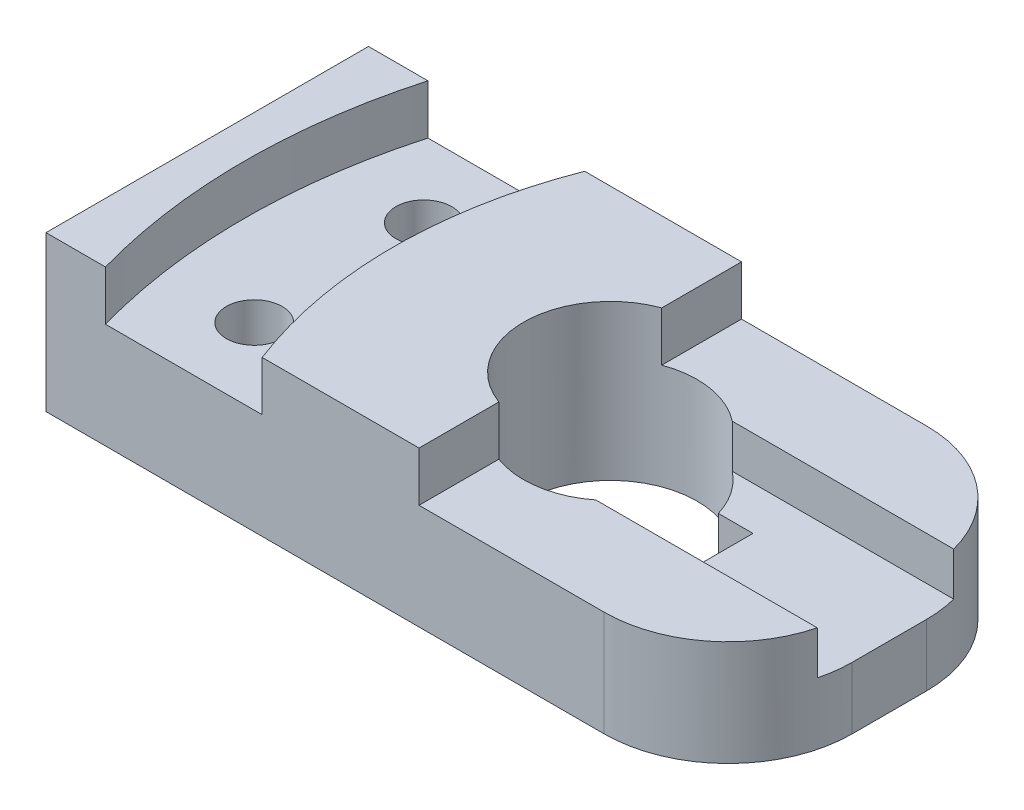
ISO-10303-21;
HEADER;
FILE_DESCRIPTION(('STEP AP214'),'2;1');
FILE_NAME('part.step','',(''),(''),'','','');
FILE_SCHEMA(('AUTOMOTIVE_DESIGN { 1 0 10303 214 1 1 1 1 }'));
ENDSEC;
DATA;
#1=APPLICATION_CONTEXT('core data for automotive mechanical design processes');
#2=APPLICATION_PROTOCOL_DEFINITION('international standard','automotive_design',2000,#1);
#3=PRODUCT_CONTEXT('',#1,'mechanical');
#4=PRODUCT('Part','Part','',(#3));
#5=PRODUCT_RELATED_PRODUCT_CATEGORY('part','',(#4));
#6=PRODUCT_DEFINITION_FORMATION('','',#4);
#7=PRODUCT_DEFINITION_CONTEXT('part definition',#1,'design');
#8=PRODUCT_DEFINITION('design','',#6,#7);
#9=PRODUCT_DEFINITION_SHAPE('','',#8);
#10=(LENGTH_UNIT() NAMED_UNIT(*) SI_UNIT(.MILLI.,.METRE.));
#11=(NAMED_UNIT(*) PLANE_ANGLE_UNIT() SI_UNIT($,.RADIAN.));
#12=(NAMED_UNIT(*) SI_UNIT($,.STERADIAN.) SOLID_ANGLE_UNIT());
#13=UNCERTAINTY_MEASURE_WITH_UNIT(LENGTH_MEASURE(1.E-05),#10,'distance_accuracy_value','');
#14=(GEOMETRIC_REPRESENTATION_CONTEXT(3) GLOBAL_UNCERTAINTY_ASSIGNED_CONTEXT((#13)) GLOBAL_UNIT_ASSIGNED_CONTEXT((#10,
#11,#12)) REPRESENTATION_CONTEXT('',''));
#15=CARTESIAN_POINT('',(0.,0.,0.));
#16=DIRECTION('',(0.,0.,1.));
#17=DIRECTION('',(1.,0.,0.));
#18=AXIS2_PLACEMENT_3D('',#15,#16,#17);
#19=CARTESIAN_POINT('',(84.,-65.5,-4.));
#20=DIRECTION('',(0.,0.,-1.));
#21=DIRECTION('',(-1.,0.,0.));
#22=AXIS2_PLACEMENT_3D('',#19,#20,#21);
#23=PLANE('',#22);
#24=DIRECTION('',(1.,0.,0.));
#25=VECTOR('',#24,1.);
#26=CARTESIAN_POINT('',(84.,-2.5,-4.));
#27=LINE('',#26,#25);
#28=CARTESIAN_POINT('',(78.4164078649987,-2.5,-4.));
#29=VERTEX_POINT('',#28);
#30=CARTESIAN_POINT('',(84.,-2.5,-4.));
#31=VERTEX_POINT('',#30);
#32=EDGE_CURVE('E212',#29,#31,#27,.T.);
#33=ORIENTED_EDGE('',*,*,#32,.F.);
#34=DIRECTION('',(0.,1.,0.));
#35=VECTOR('',#34,1.);
#36=CARTESIAN_POINT('',(78.4164078649987,-65.5,-4.));
#37=LINE('',#36,#35);
#38=CARTESIAN_POINT('',(78.4164078649987,-12.5,-4.));
#39=VERTEX_POINT('',#38);
#40=EDGE_CURVE('E213',#39,#29,#37,.T.);
#41=ORIENTED_EDGE('',*,*,#40,.F.);
#42=DIRECTION('',(1.,0.,0.));
#43=VECTOR('',#42,1.);
#44=CARTESIAN_POINT('',(0.,-12.5,-3.99999999999999));
#45=LINE('',#44,#43);
#46=CARTESIAN_POINT('',(84.,-12.5,-4.));
#47=VERTEX_POINT('',#46);
#48=EDGE_CURVE('E342',#39,#47,#45,.T.);
#49=ORIENTED_EDGE('',*,*,#48,.T.);
#50=DIRECTION('',(0.,1.,0.));
#51=VECTOR('',#50,1.);
#52=CARTESIAN_POINT('',(84.,-65.5,-4.));
#53=LINE('',#52,#51);
#54=EDGE_CURVE('E261',#47,#31,#53,.T.);
#55=ORIENTED_EDGE('',*,*,#54,.T.);
#56=EDGE_LOOP('',(#33,#41,#49,#55));
#57=FACE_BOUND('',#56,.T.);
#58=ADVANCED_FACE('F39',(#57),#23,.F.);
#59=CARTESIAN_POINT('',(84.,-65.5,4.));
#60=DIRECTION('',(1.,0.,0.));
#61=DIRECTION('',(0.,0.,-1.));
#62=AXIS2_PLACEMENT_3D('',#59,#60,#61);
#63=PLANE('',#62);
#64=DIRECTION('',(0.,0.,1.));
#65=VECTOR('',#64,1.);
#66=CARTESIAN_POINT('',(84.,-2.5,4.));
#67=LINE('',#66,#65);
#68=CARTESIAN_POINT('',(84.,-2.5,4.));
#69=VERTEX_POINT('',#68);
#70=EDGE_CURVE('E220',#31,#69,#67,.T.);
#71=ORIENTED_EDGE('',*,*,#70,.F.);
#72=ORIENTED_EDGE('',*,*,#54,.F.);
#73=DIRECTION('',(0.,0.,1.));
#74=VECTOR('',#73,1.);
#75=CARTESIAN_POINT('',(84.,-12.5,0.));
#76=LINE('',#75,#74);
#77=CARTESIAN_POINT('',(84.,-12.5,4.));
#78=VERTEX_POINT('',#77);
#79=EDGE_CURVE('E345',#47,#78,#76,.T.);
#80=ORIENTED_EDGE('',*,*,#79,.T.);
#81=DIRECTION('',(0.,1.,0.));
#82=VECTOR('',#81,1.);
#83=CARTESIAN_POINT('',(84.,-65.5,4.));
#84=LINE('',#83,#82);
#85=EDGE_CURVE('E269',#78,#69,#84,.T.);
#86=ORIENTED_EDGE('',*,*,#85,.T.);
#87=EDGE_LOOP('',(#71,#72,#80,#86));
#88=FACE_BOUND('',#87,.T.);
#89=ADVANCED_FACE('F445',(#88),#63,.F.);
#90=CARTESIAN_POINT('',(84.,-65.5,4.));
#91=DIRECTION('',(0.,0.,-1.));
#92=DIRECTION('',(-1.,0.,0.));
#93=AXIS2_PLACEMENT_3D('',#90,#91,#92);
#94=PLANE('',#93);
#95=DIRECTION('',(0.,1.,0.));
#96=VECTOR('',#95,1.);
#97=CARTESIAN_POINT('',(78.4164078649987,-65.5,4.));
#98=LINE('',#97,#96);
#99=CARTESIAN_POINT('',(78.4164078649987,-12.5,4.00000000000001));
#100=VERTEX_POINT('',#99);
#101=CARTESIAN_POINT('',(78.4164078649987,-2.5,4.));
#102=VERTEX_POINT('',#101);
#103=EDGE_CURVE('E272',#100,#102,#98,.T.);
#104=ORIENTED_EDGE('',*,*,#103,.T.);
#105=DIRECTION('',(-1.,0.,0.));
#106=VECTOR('',#105,1.);
#107=CARTESIAN_POINT('',(78.4164078649987,-2.5,4.));
#108=LINE('',#107,#106);
#109=EDGE_CURVE('E222',#69,#102,#108,.T.);
#110=ORIENTED_EDGE('',*,*,#109,.F.);
#111=ORIENTED_EDGE('',*,*,#85,.F.);
#112=DIRECTION('',(1.,0.,0.));
#113=VECTOR('',#112,1.);
#114=CARTESIAN_POINT('',(0.,-12.5,4.00000000000001));
#115=LINE('',#114,#113);
#116=EDGE_CURVE('E338',#100,#78,#115,.T.);
#117=ORIENTED_EDGE('',*,*,#116,.F.);
#118=EDGE_LOOP('',(#104,#110,#111,#117));
#119=FACE_BOUND('',#118,.T.);
#120=ADVANCED_FACE('F449',(#119),#94,.T.);
#121=CARTESIAN_POINT('',(0.,12.5,26.));
#122=DIRECTION('',(0.,0.,-1.));
#123=DIRECTION('',(-1.,0.,0.));
#124=AXIS2_PLACEMENT_3D('',#121,#122,#123);
#125=PLANE('',#124);
#126=DIRECTION('',(1.,0.,0.));
#127=VECTOR('',#126,1.);
#128=CARTESIAN_POINT('',(0.,-12.5,26.));
#129=LINE('',#128,#127);
#130=CARTESIAN_POINT('',(0.,-12.5,26.));
#131=VERTEX_POINT('',#130);
#132=CARTESIAN_POINT('',(90.,-12.5,26.));
#133=VERTEX_POINT('',#132);
#134=EDGE_CURVE('E318',#131,#133,#129,.T.);
#135=ORIENTED_EDGE('',*,*,#134,.T.);
#136=DIRECTION('',(0.,-1.,0.));
#137=VECTOR('',#136,1.);
#138=CARTESIAN_POINT('',(90.,12.5,26.));
#139=LINE('',#138,#137);
#140=CARTESIAN_POINT('',(90.,4.5,26.));
#141=VERTEX_POINT('',#140);
#142=EDGE_CURVE('E64',#133,#141,#139,.F.);
#143=ORIENTED_EDGE('',*,*,#142,.T.);
#144=DIRECTION('',(1.,0.,0.));
#145=VECTOR('',#144,1.);
#146=CARTESIAN_POINT('',(110.,4.5,26.));
#147=LINE('',#146,#145);
#148=CARTESIAN_POINT('',(60.1523600510817,4.5,26.));
#149=VERTEX_POINT('',#148);
#150=EDGE_CURVE('E260',#149,#141,#147,.T.);
#151=ORIENTED_EDGE('',*,*,#150,.F.);
#152=DIRECTION('',(0.,1.,0.));
#153=VECTOR('',#152,1.);
#154=CARTESIAN_POINT('',(60.1523600510817,4.5,26.));
#155=LINE('',#154,#153);
#156=CARTESIAN_POINT('',(60.1523600510817,12.5,26.));
#157=VERTEX_POINT('',#156);
#158=EDGE_CURVE('E250',#149,#157,#155,.T.);
#159=ORIENTED_EDGE('',*,*,#158,.T.);
#160=DIRECTION('',(1.,0.,0.));
#161=VECTOR('',#160,1.);
#162=CARTESIAN_POINT('',(0.,12.5,26.));
#163=LINE('',#162,#161);
#164=CARTESIAN_POINT('',(34.8583586736219,12.5,26.));
#165=VERTEX_POINT('',#164);
#166=EDGE_CURVE('E308',#165,#157,#163,.T.);
#167=ORIENTED_EDGE('',*,*,#166,.F.);
#168=DIRECTION('',(0.,1.,0.));
#169=VECTOR('',#168,1.);
#170=CARTESIAN_POINT('',(34.8583586736219,4.5,26.));
#171=LINE('',#170,#169);
#172=CARTESIAN_POINT('',(34.8583586736219,4.5,26.));
#173=VERTEX_POINT('',#172);
#174=EDGE_CURVE('E294',#173,#165,#171,.T.);
#175=ORIENTED_EDGE('',*,*,#174,.F.);
#176=DIRECTION('',(1.,0.,0.));
#177=VECTOR('',#176,1.);
#178=CARTESIAN_POINT('',(9.58787958281658,4.5,26.));
#179=LINE('',#178,#177);
#180=CARTESIAN_POINT('',(9.58787958281658,4.5,26.));
#181=VERTEX_POINT('',#180);
#182=EDGE_CURVE('E282',#181,#173,#179,.T.);
#183=ORIENTED_EDGE('',*,*,#182,.F.);
#184=DIRECTION('',(0.,1.,0.));
#185=VECTOR('',#184,1.);
#186=CARTESIAN_POINT('',(9.58787958281658,4.5,26.));
#187=LINE('',#186,#185);
#188=CARTESIAN_POINT('',(9.58787958281658,12.5,26.));
#189=VERTEX_POINT('',#188);
#190=EDGE_CURVE('E292',#181,#189,#187,.T.);
#191=ORIENTED_EDGE('',*,*,#190,.T.);
#192=CARTESIAN_POINT('',(0.,12.5,26.));
#193=VERTEX_POINT('',#192);
#194=EDGE_CURVE('E309',#193,#189,#163,.T.);
#195=ORIENTED_EDGE('',*,*,#194,.F.);
#196=DIRECTION('',(0.,-1.,0.));
#197=VECTOR('',#196,1.);
#198=CARTESIAN_POINT('',(0.,12.5,26.));
#199=LINE('',#198,#197);
#200=EDGE_CURVE('E326',#193,#131,#199,.T.);
#201=ORIENTED_EDGE('',*,*,#200,.T.);
#202=EDGE_LOOP('',(#135,#143,#151,#159,#167,#175,#183,#191,#195,#201));
#203=FACE_BOUND('',#202,.T.);
#204=ADVANCED_FACE('F392',(#203),#125,.F.);
#205=CARTESIAN_POINT('',(0.,12.5,-26.));
#206=DIRECTION('',(0.,0.,1.));
#207=DIRECTION('',(1.,0.,0.));
#208=AXIS2_PLACEMENT_3D('',#205,#206,#207);
#209=PLANE('',#208);
#210=DIRECTION('',(-1.,0.,0.));
#211=VECTOR('',#210,1.);
#212=CARTESIAN_POINT('',(60.1523600510817,4.5,-26.));
#213=LINE('',#212,#211);
#214=CARTESIAN_POINT('',(90.,4.5,-26.));
#215=VERTEX_POINT('',#214);
#216=CARTESIAN_POINT('',(60.1523600510817,4.5,-26.));
#217=VERTEX_POINT('',#216);
#218=EDGE_CURVE('E233',#215,#217,#213,.T.);
#219=ORIENTED_EDGE('',*,*,#218,.F.);
#220=DIRECTION('',(0.,-1.,0.));
#221=VECTOR('',#220,1.);
#222=CARTESIAN_POINT('',(90.,12.5,-26.));
#223=LINE('',#222,#221);
#224=CARTESIAN_POINT('',(90.,-12.5,-26.));
#225=VERTEX_POINT('',#224);
#226=EDGE_CURVE('E350',#215,#225,#223,.T.);
#227=ORIENTED_EDGE('',*,*,#226,.T.);
#228=DIRECTION('',(-1.,0.,0.));
#229=VECTOR('',#228,1.);
#230=CARTESIAN_POINT('',(0.,-12.5,-26.));
#231=LINE('',#230,#229);
#232=CARTESIAN_POINT('',(0.,-12.5,-26.));
#233=VERTEX_POINT('',#232);
#234=EDGE_CURVE('E307',#225,#233,#231,.T.);
#235=ORIENTED_EDGE('',*,*,#234,.T.);
#236=DIRECTION('',(0.,-1.,0.));
#237=VECTOR('',#236,1.);
#238=CARTESIAN_POINT('',(0.,12.5,-26.));
#239=LINE('',#238,#237);
#240=CARTESIAN_POINT('',(0.,12.5,-26.));
#241=VERTEX_POINT('',#240);
#242=EDGE_CURVE('E317',#241,#233,#239,.T.);
#243=ORIENTED_EDGE('',*,*,#242,.F.);
#244=DIRECTION('',(-1.,0.,0.));
#245=VECTOR('',#244,1.);
#246=CARTESIAN_POINT('',(0.,12.5,-26.));
#247=LINE('',#246,#245);
#248=CARTESIAN_POINT('',(9.58787958281658,12.5,-26.));
#249=VERTEX_POINT('',#248);
#250=EDGE_CURVE('E312',#249,#241,#247,.T.);
#251=ORIENTED_EDGE('',*,*,#250,.F.);
#252=DIRECTION('',(0.,1.,0.));
#253=VECTOR('',#252,1.);
#254=CARTESIAN_POINT('',(9.58787958281659,4.5,-26.));
#255=LINE('',#254,#253);
#256=CARTESIAN_POINT('',(9.58787958281659,4.5,-26.));
#257=VERTEX_POINT('',#256);
#258=EDGE_CURVE('E287',#257,#249,#255,.T.);
#259=ORIENTED_EDGE('',*,*,#258,.F.);
#260=DIRECTION('',(1.,0.,0.));
#261=VECTOR('',#260,1.);
#262=CARTESIAN_POINT('',(9.58787958281658,4.5,-26.));
#263=LINE('',#262,#261);
#264=CARTESIAN_POINT('',(34.8583586736219,4.5,-26.));
#265=VERTEX_POINT('',#264);
#266=EDGE_CURVE('E273',#257,#265,#263,.T.);
#267=ORIENTED_EDGE('',*,*,#266,.T.);
#268=DIRECTION('',(0.,1.,0.));
#269=VECTOR('',#268,1.);
#270=CARTESIAN_POINT('',(34.8583586736219,4.5,-26.));
#271=LINE('',#270,#269);
#272=CARTESIAN_POINT('',(34.8583586736219,12.5,-26.));
#273=VERTEX_POINT('',#272);
#274=EDGE_CURVE('E300',#265,#273,#271,.T.);
#275=ORIENTED_EDGE('',*,*,#274,.T.);
#276=CARTESIAN_POINT('',(60.1523600510817,12.5,-26.));
#277=VERTEX_POINT('',#276);
#278=EDGE_CURVE('E313',#277,#273,#247,.T.);
#279=ORIENTED_EDGE('',*,*,#278,.F.);
#280=DIRECTION('',(0.,1.,0.));
#281=VECTOR('',#280,1.);
#282=CARTESIAN_POINT('',(60.1523600510817,4.5,-26.));
#283=LINE('',#282,#281);
#284=EDGE_CURVE('E237',#217,#277,#283,.T.);
#285=ORIENTED_EDGE('',*,*,#284,.F.);
#286=EDGE_LOOP('',(#219,#227,#235,#243,#251,#259,#267,#275,#279,#285));
#287=FACE_BOUND('',#286,.T.);
#288=ADVANCED_FACE('F374',(#287),#209,.F.);
#289=CARTESIAN_POINT('',(0.,12.5,0.));
#290=DIRECTION('',(0.,-1.,0.));
#291=DIRECTION('',(0.,0.,-1.));
#292=AXIS2_PLACEMENT_3D('',#289,#290,#291);
#293=PLANE('',#292);
#294=CARTESIAN_POINT('',(65.,12.5,0.));
#295=DIRECTION('',(0.,1.,0.));
#296=DIRECTION('',(0.,0.,1.));
#297=AXIS2_PLACEMENT_3D('',#294,#295,#296);
#298=CIRCLE('',#297,14.);
#299=CARTESIAN_POINT('',(60.1523600510817,12.5,-13.1339402665632));
#300=VERTEX_POINT('',#299);
#301=CARTESIAN_POINT('',(60.1523600510817,12.5,13.1339402665632));
#302=VERTEX_POINT('',#301);
#303=EDGE_CURVE('E244',#300,#302,#298,.T.);
#304=ORIENTED_EDGE('',*,*,#303,.F.);
#305=DIRECTION('',(0.,0.,1.));
#306=VECTOR('',#305,1.);
#307=CARTESIAN_POINT('',(60.1523600510817,12.5,-26.));
#308=LINE('',#307,#306);
#309=EDGE_CURVE('E234',#277,#300,#308,.T.);
#310=ORIENTED_EDGE('',*,*,#309,.F.);
#311=ORIENTED_EDGE('',*,*,#278,.T.);
#312=CARTESIAN_POINT('',(102.,12.5,0.));
#313=DIRECTION('',(0.,1.,0.));
#314=DIRECTION('',(0.,0.,1.));
#315=AXIS2_PLACEMENT_3D('',#312,#313,#314);
#316=CIRCLE('',#315,72.);
#317=EDGE_CURVE('E267',#273,#165,#316,.T.);
#318=ORIENTED_EDGE('',*,*,#317,.T.);
#319=ORIENTED_EDGE('',*,*,#166,.T.);
#320=DIRECTION('',(0.,0.,1.));
#321=VECTOR('',#320,1.);
#322=CARTESIAN_POINT('',(60.1523600510817,12.5,13.1339402665632));
#323=LINE('',#322,#321);
#324=EDGE_CURVE('E241',#302,#157,#323,.T.);
#325=ORIENTED_EDGE('',*,*,#324,.F.);
#326=EDGE_LOOP('',(#304,#310,#311,#318,#319,#325));
#327=FACE_BOUND('',#326,.T.);
#328=ADVANCED_FACE('F419',(#327),#293,.F.);
#329=CARTESIAN_POINT('',(21.0741079752592,-62.5,-13.8497805558295));
#330=DIRECTION('',(0.,1.,0.));
#331=DIRECTION('',(0.,0.,1.));
#332=AXIS2_PLACEMENT_3D('',#329,#330,#331);
#333=CYLINDRICAL_SURFACE('',#332,4.5);
#334=CARTESIAN_POINT('',(21.0741079752592,-12.5,-13.8497805558295));
#335=DIRECTION('',(0.,-1.,0.));
#336=DIRECTION('',(0.,0.,-1.));
#337=AXIS2_PLACEMENT_3D('',#334,#335,#336);
#338=CIRCLE('',#337,4.5);
#339=CARTESIAN_POINT('',(21.0741079752592,-12.5,-18.3497805558295));
#340=VERTEX_POINT('',#339);
#341=EDGE_CURVE('E302',#340,#340,#338,.T.);
#342=ORIENTED_EDGE('',*,*,#341,.T.);
#343=EDGE_LOOP('',(#342));
#344=FACE_BOUND('',#343,.T.);
#345=CARTESIAN_POINT('',(21.0741079752592,4.5,-13.8497805558295));
#346=DIRECTION('',(0.,1.,0.));
#347=DIRECTION('',(0.,0.,1.));
#348=AXIS2_PLACEMENT_3D('',#345,#346,#347);
#349=CIRCLE('',#348,4.5);
#350=CARTESIAN_POINT('',(21.0741079752592,4.5,-9.34978055582945));
#351=VERTEX_POINT('',#350);
#352=EDGE_CURVE('E301',#351,#351,#349,.F.);
#353=ORIENTED_EDGE('',*,*,#352,.F.);
#354=EDGE_LOOP('',(#353));
#355=FACE_BOUND('',#354,.T.);
#356=ADVANCED_FACE('F464',(#344,#355),#333,.F.);
#357=CARTESIAN_POINT('',(21.3438782276735,-62.5,13.7647223219684));
#358=DIRECTION('',(0.,1.,0.));
#359=DIRECTION('',(0.,0.,1.));
#360=AXIS2_PLACEMENT_3D('',#357,#358,#359);
#361=CYLINDRICAL_SURFACE('',#360,4.5);
#362=CARTESIAN_POINT('',(21.3438782276735,-12.5,13.7647223219684));
#363=DIRECTION('',(0.,-1.,0.));
#364=DIRECTION('',(0.,0.,-1.));
#365=AXIS2_PLACEMENT_3D('',#362,#363,#364);
#366=CIRCLE('',#365,4.5);
#367=CARTESIAN_POINT('',(21.3438782276735,-12.5,9.26472232196836));
#368=VERTEX_POINT('',#367);
#369=EDGE_CURVE('E324',#368,#368,#366,.T.);
#370=ORIENTED_EDGE('',*,*,#369,.T.);
#371=EDGE_LOOP('',(#370));
#372=FACE_BOUND('',#371,.T.);
#373=CARTESIAN_POINT('',(21.3438782276735,4.5,13.7647223219684));
#374=DIRECTION('',(0.,1.,0.));
#375=DIRECTION('',(0.,0.,1.));
#376=AXIS2_PLACEMENT_3D('',#373,#374,#375);
#377=CIRCLE('',#376,4.5);
#378=CARTESIAN_POINT('',(21.3438782276735,4.5,18.2647223219684));
#379=VERTEX_POINT('',#378);
#380=EDGE_CURVE('E297',#379,#379,#377,.F.);
#381=ORIENTED_EDGE('',*,*,#380,.F.);
#382=EDGE_LOOP('',(#381));
#383=FACE_BOUND('',#382,.T.);
#384=ADVANCED_FACE('F458',(#372,#383),#361,.F.);
#385=CARTESIAN_POINT('',(0.,12.5,26.));
#386=DIRECTION('',(1.,0.,0.));
#387=DIRECTION('',(0.,0.,-1.));
#388=AXIS2_PLACEMENT_3D('',#385,#386,#387);
#389=PLANE('',#388);
#390=DIRECTION('',(0.,0.,1.));
#391=VECTOR('',#390,1.);
#392=CARTESIAN_POINT('',(0.,-12.5,26.));
#393=LINE('',#392,#391);
#394=EDGE_CURVE('E320',#233,#131,#393,.T.);
#395=ORIENTED_EDGE('',*,*,#394,.T.);
#396=ORIENTED_EDGE('',*,*,#200,.F.);
#397=DIRECTION('',(0.,0.,1.));
#398=VECTOR('',#397,1.);
#399=CARTESIAN_POINT('',(0.,12.5,26.));
#400=LINE('',#399,#398);
#401=EDGE_CURVE('E304',#241,#193,#400,.T.);
#402=ORIENTED_EDGE('',*,*,#401,.F.);
#403=ORIENTED_EDGE('',*,*,#242,.T.);
#404=EDGE_LOOP('',(#395,#396,#402,#403));
#405=FACE_BOUND('',#404,.T.);
#406=ADVANCED_FACE('F393',(#405),#389,.F.);
#407=CARTESIAN_POINT('',(110.,12.5,26.));
#408=DIRECTION('',(-1.,0.,0.));
#409=DIRECTION('',(0.,0.,1.));
#410=AXIS2_PLACEMENT_3D('',#407,#408,#409);
#411=PLANE('',#410);
#412=DIRECTION('',(0.,0.,-1.));
#413=VECTOR('',#412,1.);
#414=CARTESIAN_POINT('',(110.,-12.5,26.));
#415=LINE('',#414,#413);
#416=CARTESIAN_POINT('',(110.,-12.5,6.00000000000001));
#417=VERTEX_POINT('',#416);
#418=CARTESIAN_POINT('',(110.,-12.5,-5.99999999999998));
#419=VERTEX_POINT('',#418);
#420=EDGE_CURVE('E325',#417,#419,#415,.T.);
#421=ORIENTED_EDGE('',*,*,#420,.T.);
#422=DIRECTION('',(0.,-1.,0.));
#423=VECTOR('',#422,1.);
#424=CARTESIAN_POINT('',(110.,12.5,-6.));
#425=LINE('',#424,#423);
#426=CARTESIAN_POINT('',(110.,-2.5,-6.));
#427=VERTEX_POINT('',#426);
#428=EDGE_CURVE('E357',#419,#427,#425,.F.);
#429=ORIENTED_EDGE('',*,*,#428,.T.);
#430=DIRECTION('',(0.,0.,-1.));
#431=VECTOR('',#430,1.);
#432=CARTESIAN_POINT('',(110.,-2.5,-11.));
#433=LINE('',#432,#431);
#434=CARTESIAN_POINT('',(110.,-2.5,6.));
#435=VERTEX_POINT('',#434);
#436=EDGE_CURVE('E199',#435,#427,#433,.T.);
#437=ORIENTED_EDGE('',*,*,#436,.F.);
#438=DIRECTION('',(0.,-1.,0.));
#439=VECTOR('',#438,1.);
#440=CARTESIAN_POINT('',(110.,12.5,6.));
#441=LINE('',#440,#439);
#442=EDGE_CURVE('E353',#435,#417,#441,.T.);
#443=ORIENTED_EDGE('',*,*,#442,.T.);
#444=EDGE_LOOP('',(#421,#429,#437,#443));
#445=FACE_BOUND('',#444,.T.);
#446=ADVANCED_FACE('F383',(#445),#411,.F.);
#447=ORIENTED_EDGE('',*,*,#194,.T.);
#448=CARTESIAN_POINT('',(102.,12.5,0.));
#449=DIRECTION('',(0.,1.,0.));
#450=DIRECTION('',(0.,0.,1.));
#451=AXIS2_PLACEMENT_3D('',#448,#449,#450);
#452=CIRCLE('',#451,96.);
#453=EDGE_CURVE('E278',#249,#189,#452,.T.);
#454=ORIENTED_EDGE('',*,*,#453,.F.);
#455=ORIENTED_EDGE('',*,*,#250,.T.);
#456=ORIENTED_EDGE('',*,*,#401,.T.);
#457=EDGE_LOOP('',(#447,#454,#455,#456));
#458=FACE_BOUND('',#457,.T.);
#459=ADVANCED_FACE('F402',(#458),#293,.F.);
#460=CARTESIAN_POINT('',(0.,-12.5,0.));
#461=DIRECTION('',(0.,-1.,0.));
#462=DIRECTION('',(0.,0.,-1.));
#463=AXIS2_PLACEMENT_3D('',#460,#461,#462);
#464=PLANE('',#463);
#465=ORIENTED_EDGE('',*,*,#48,.F.);
#466=CARTESIAN_POINT('',(65.,-12.5,0.));
#467=DIRECTION('',(0.,-1.,0.));
#468=DIRECTION('',(0.,0.,-1.));
#469=AXIS2_PLACEMENT_3D('',#466,#467,#468);
#470=CIRCLE('',#469,14.);
#471=EDGE_CURVE('E332',#100,#39,#470,.T.);
#472=ORIENTED_EDGE('',*,*,#471,.F.);
#473=ORIENTED_EDGE('',*,*,#116,.T.);
#474=ORIENTED_EDGE('',*,*,#79,.F.);
#475=EDGE_LOOP('',(#465,#472,#473,#474));
#476=FACE_BOUND('',#475,.T.);
#477=ORIENTED_EDGE('',*,*,#369,.F.);
#478=EDGE_LOOP('',(#477));
#479=FACE_BOUND('',#478,.T.);
#480=ORIENTED_EDGE('',*,*,#341,.F.);
#481=EDGE_LOOP('',(#480));
#482=FACE_BOUND('',#481,.T.);
#483=ORIENTED_EDGE('',*,*,#234,.F.);
#484=CARTESIAN_POINT('',(90.,-12.5,-6.));
#485=DIRECTION('',(0.,-1.,0.));
#486=DIRECTION('',(0.,0.,-1.));
#487=AXIS2_PLACEMENT_3D('',#484,#485,#486);
#488=CIRCLE('',#487,20.);
#489=EDGE_CURVE('E352',#225,#419,#488,.T.);
#490=ORIENTED_EDGE('',*,*,#489,.T.);
#491=ORIENTED_EDGE('',*,*,#420,.F.);
#492=CARTESIAN_POINT('',(90.,-12.5,6.));
#493=DIRECTION('',(0.,-1.,0.));
#494=DIRECTION('',(0.,0.,-1.));
#495=AXIS2_PLACEMENT_3D('',#492,#493,#494);
#496=CIRCLE('',#495,20.);
#497=EDGE_CURVE('E348',#417,#133,#496,.T.);
#498=ORIENTED_EDGE('',*,*,#497,.T.);
#499=ORIENTED_EDGE('',*,*,#134,.F.);
#500=ORIENTED_EDGE('',*,*,#394,.F.);
#501=EDGE_LOOP('',(#483,#490,#491,#498,#499,#500));
#502=FACE_BOUND('',#501,.T.);
#503=ADVANCED_FACE('F385',(#476,#479,#482,#502),#464,.T.);
#504=CARTESIAN_POINT('',(102.,4.5,0.));
#505=DIRECTION('',(0.,1.,0.));
#506=DIRECTION('',(0.,0.,1.));
#507=AXIS2_PLACEMENT_3D('',#504,#505,#506);
#508=PLANE('',#507);
#509=ORIENTED_EDGE('',*,*,#266,.F.);
#510=CARTESIAN_POINT('',(102.,4.5,0.));
#511=DIRECTION('',(0.,1.,0.));
#512=DIRECTION('',(0.,0.,1.));
#513=AXIS2_PLACEMENT_3D('',#510,#511,#512);
#514=CIRCLE('',#513,96.);
#515=EDGE_CURVE('E281',#257,#181,#514,.T.);
#516=ORIENTED_EDGE('',*,*,#515,.T.);
#517=ORIENTED_EDGE('',*,*,#182,.T.);
#518=CARTESIAN_POINT('',(102.,4.5,0.));
#519=DIRECTION('',(0.,1.,0.));
#520=DIRECTION('',(0.,0.,1.));
#521=AXIS2_PLACEMENT_3D('',#518,#519,#520);
#522=CIRCLE('',#521,72.);
#523=EDGE_CURVE('E280',#265,#173,#522,.T.);
#524=ORIENTED_EDGE('',*,*,#523,.F.);
#525=EDGE_LOOP('',(#509,#516,#517,#524));
#526=FACE_BOUND('',#525,.T.);
#527=ORIENTED_EDGE('',*,*,#380,.T.);
#528=EDGE_LOOP('',(#527));
#529=FACE_BOUND('',#528,.T.);
#530=ORIENTED_EDGE('',*,*,#352,.T.);
#531=EDGE_LOOP('',(#530));
#532=FACE_BOUND('',#531,.T.);
#533=ADVANCED_FACE('F408',(#526,#529,#532),#508,.T.);
#534=CARTESIAN_POINT('',(102.,4.5,0.));
#535=DIRECTION('',(0.,1.,0.));
#536=DIRECTION('',(0.,0.,1.));
#537=AXIS2_PLACEMENT_3D('',#534,#535,#536);
#538=CYLINDRICAL_SURFACE('',#537,72.);
#539=ORIENTED_EDGE('',*,*,#317,.F.);
#540=ORIENTED_EDGE('',*,*,#274,.F.);
#541=ORIENTED_EDGE('',*,*,#523,.T.);
#542=ORIENTED_EDGE('',*,*,#174,.T.);
#543=EDGE_LOOP('',(#539,#540,#541,#542));
#544=FACE_BOUND('',#543,.T.);
#545=ADVANCED_FACE('F411',(#544),#538,.T.);
#546=CARTESIAN_POINT('',(102.,4.5,0.));
#547=DIRECTION('',(0.,1.,0.));
#548=DIRECTION('',(0.,0.,1.));
#549=AXIS2_PLACEMENT_3D('',#546,#547,#548);
#550=CYLINDRICAL_SURFACE('',#549,96.);
#551=ORIENTED_EDGE('',*,*,#453,.T.);
#552=ORIENTED_EDGE('',*,*,#190,.F.);
#553=ORIENTED_EDGE('',*,*,#515,.F.);
#554=ORIENTED_EDGE('',*,*,#258,.T.);
#555=EDGE_LOOP('',(#551,#552,#553,#554));
#556=FACE_BOUND('',#555,.T.);
#557=ADVANCED_FACE('F401',(#556),#550,.F.);
#558=CARTESIAN_POINT('',(65.,-65.5,0.));
#559=DIRECTION('',(0.,1.,0.));
#560=DIRECTION('',(0.,0.,1.));
#561=AXIS2_PLACEMENT_3D('',#558,#559,#560);
#562=CYLINDRICAL_SURFACE('',#561,14.);
#563=CARTESIAN_POINT('',(65.,-2.5,0.));
#564=DIRECTION('',(0.,-1.,0.));
#565=DIRECTION('',(0.,0.,1.));
#566=AXIS2_PLACEMENT_3D('',#563,#564,#565);
#567=CIRCLE('',#566,14.);
#568=CARTESIAN_POINT('',(73.6602540378444,-2.5,-11.));
#569=VERTEX_POINT('',#568);
#570=EDGE_CURVE('E191',#569,#29,#567,.T.);
#571=ORIENTED_EDGE('',*,*,#570,.F.);
#572=DIRECTION('',(0.,1.,0.));
#573=VECTOR('',#572,1.);
#574=CARTESIAN_POINT('',(73.6602540378444,-2.5,-11.));
#575=LINE('',#574,#573);
#576=CARTESIAN_POINT('',(73.6602540378444,4.5,-11.));
#577=VERTEX_POINT('',#576);
#578=EDGE_CURVE('E201',#569,#577,#575,.T.);
#579=ORIENTED_EDGE('',*,*,#578,.T.);
#580=CARTESIAN_POINT('',(65.,4.5,0.));
#581=DIRECTION('',(0.,-1.,0.));
#582=DIRECTION('',(0.,0.,1.));
#583=AXIS2_PLACEMENT_3D('',#580,#581,#582);
#584=CIRCLE('',#583,14.);
#585=CARTESIAN_POINT('',(60.1523600510817,4.5,-13.1339402665632));
#586=VERTEX_POINT('',#585);
#587=EDGE_CURVE('E236',#586,#577,#584,.T.);
#588=ORIENTED_EDGE('',*,*,#587,.F.);
#589=DIRECTION('',(0.,1.,0.));
#590=VECTOR('',#589,1.);
#591=CARTESIAN_POINT('',(60.1523600510817,4.5,-13.1339402665632));
#592=LINE('',#591,#590);
#593=EDGE_CURVE('E245',#586,#300,#592,.T.);
#594=ORIENTED_EDGE('',*,*,#593,.T.);
#595=ORIENTED_EDGE('',*,*,#303,.T.);
#596=DIRECTION('',(0.,1.,0.));
#597=VECTOR('',#596,1.);
#598=CARTESIAN_POINT('',(60.1523600510817,4.5,13.1339402665632));
#599=LINE('',#598,#597);
#600=CARTESIAN_POINT('',(60.1523600510817,4.5,13.1339402665632));
#601=VERTEX_POINT('',#600);
#602=EDGE_CURVE('E230',#601,#302,#599,.T.);
#603=ORIENTED_EDGE('',*,*,#602,.F.);
#604=CARTESIAN_POINT('',(65.,4.5,0.));
#605=DIRECTION('',(0.,-1.,0.));
#606=DIRECTION('',(0.,0.,1.));
#607=AXIS2_PLACEMENT_3D('',#604,#605,#606);
#608=CIRCLE('',#607,14.);
#609=CARTESIAN_POINT('',(73.6602540378444,4.5,11.));
#610=VERTEX_POINT('',#609);
#611=EDGE_CURVE('E249',#610,#601,#608,.T.);
#612=ORIENTED_EDGE('',*,*,#611,.F.);
#613=DIRECTION('',(0.,1.,0.));
#614=VECTOR('',#613,1.);
#615=CARTESIAN_POINT('',(73.6602540378444,-2.5,11.));
#616=LINE('',#615,#614);
#617=CARTESIAN_POINT('',(73.6602540378444,-2.5,11.));
#618=VERTEX_POINT('',#617);
#619=EDGE_CURVE('E206',#618,#610,#616,.T.);
#620=ORIENTED_EDGE('',*,*,#619,.F.);
#621=CARTESIAN_POINT('',(65.,-2.5,0.));
#622=DIRECTION('',(0.,-1.,0.));
#623=DIRECTION('',(0.,0.,1.));
#624=AXIS2_PLACEMENT_3D('',#621,#622,#623);
#625=CIRCLE('',#624,14.);
#626=EDGE_CURVE('E223',#102,#618,#625,.T.);
#627=ORIENTED_EDGE('',*,*,#626,.F.);
#628=ORIENTED_EDGE('',*,*,#103,.F.);
#629=ORIENTED_EDGE('',*,*,#471,.T.);
#630=ORIENTED_EDGE('',*,*,#40,.T.);
#631=EDGE_LOOP('',(#571,#579,#588,#594,#595,#603,#612,#620,#627,#628,#629,#630));
#632=FACE_BOUND('',#631,.T.);
#633=ADVANCED_FACE('F211',(#632),#562,.F.);
#634=CARTESIAN_POINT('',(60.1523600510817,4.5,13.1339402665632));
#635=DIRECTION('',(-1.,0.,0.));
#636=DIRECTION('',(0.,0.,1.));
#637=AXIS2_PLACEMENT_3D('',#634,#635,#636);
#638=PLANE('',#637);
#639=ORIENTED_EDGE('',*,*,#324,.T.);
#640=ORIENTED_EDGE('',*,*,#158,.F.);
#641=DIRECTION('',(0.,0.,1.));
#642=VECTOR('',#641,1.);
#643=CARTESIAN_POINT('',(60.1523600510817,4.5,13.1339402665632));
#644=LINE('',#643,#642);
#645=EDGE_CURVE('E254',#601,#149,#644,.T.);
#646=ORIENTED_EDGE('',*,*,#645,.F.);
#647=ORIENTED_EDGE('',*,*,#602,.T.);
#648=EDGE_LOOP('',(#639,#640,#646,#647));
#649=FACE_BOUND('',#648,.T.);
#650=ADVANCED_FACE('F422',(#649),#638,.F.);
#651=CARTESIAN_POINT('',(65.,4.5,0.));
#652=DIRECTION('',(0.,1.,0.));
#653=DIRECTION('',(0.,0.,1.));
#654=AXIS2_PLACEMENT_3D('',#651,#652,#653);
#655=PLANE('',#654);
#656=ORIENTED_EDGE('',*,*,#150,.T.);
#657=CARTESIAN_POINT('',(90.,4.5,6.));
#658=DIRECTION('',(0.,1.,0.));
#659=DIRECTION('',(0.,0.,1.));
#660=AXIS2_PLACEMENT_3D('',#657,#658,#659);
#661=CIRCLE('',#660,20.);
#662=CARTESIAN_POINT('',(109.364916731037,4.5,11.));
#663=VERTEX_POINT('',#662);
#664=EDGE_CURVE('E50',#141,#663,#661,.T.);
#665=ORIENTED_EDGE('',*,*,#664,.T.);
#666=DIRECTION('',(-1.,0.,0.));
#667=VECTOR('',#666,1.);
#668=CARTESIAN_POINT('',(73.6602540378444,4.5,11.));
#669=LINE('',#668,#667);
#670=EDGE_CURVE('E259',#663,#610,#669,.T.);
#671=ORIENTED_EDGE('',*,*,#670,.T.);
#672=ORIENTED_EDGE('',*,*,#611,.T.);
#673=ORIENTED_EDGE('',*,*,#645,.T.);
#674=EDGE_LOOP('',(#656,#665,#671,#672,#673));
#675=FACE_BOUND('',#674,.T.);
#676=ADVANCED_FACE('F421',(#675),#655,.T.);
#677=CARTESIAN_POINT('',(60.1523600510817,4.5,-26.));
#678=DIRECTION('',(-1.,0.,0.));
#679=DIRECTION('',(0.,0.,1.));
#680=AXIS2_PLACEMENT_3D('',#677,#678,#679);
#681=PLANE('',#680);
#682=ORIENTED_EDGE('',*,*,#309,.T.);
#683=ORIENTED_EDGE('',*,*,#593,.F.);
#684=DIRECTION('',(0.,0.,1.));
#685=VECTOR('',#684,1.);
#686=CARTESIAN_POINT('',(60.1523600510817,4.5,-26.));
#687=LINE('',#686,#685);
#688=EDGE_CURVE('E231',#217,#586,#687,.T.);
#689=ORIENTED_EDGE('',*,*,#688,.F.);
#690=ORIENTED_EDGE('',*,*,#284,.T.);
#691=EDGE_LOOP('',(#682,#683,#689,#690));
#692=FACE_BOUND('',#691,.T.);
#693=ADVANCED_FACE('F429',(#692),#681,.F.);
#694=CARTESIAN_POINT('',(65.,4.5,0.));
#695=DIRECTION('',(0.,1.,0.));
#696=DIRECTION('',(0.,0.,1.));
#697=AXIS2_PLACEMENT_3D('',#694,#695,#696);
#698=PLANE('',#697);
#699=DIRECTION('',(1.,0.,0.));
#700=VECTOR('',#699,1.);
#701=CARTESIAN_POINT('',(73.6602540378444,4.5,-11.));
#702=LINE('',#701,#700);
#703=CARTESIAN_POINT('',(109.364916731037,4.5,-11.));
#704=VERTEX_POINT('',#703);
#705=EDGE_CURVE('E203',#577,#704,#702,.T.);
#706=ORIENTED_EDGE('',*,*,#705,.T.);
#707=CARTESIAN_POINT('',(90.,4.5,-6.));
#708=DIRECTION('',(0.,1.,0.));
#709=DIRECTION('',(0.,0.,1.));
#710=AXIS2_PLACEMENT_3D('',#707,#708,#709);
#711=CIRCLE('',#710,20.);
#712=EDGE_CURVE('E364',#704,#215,#711,.T.);
#713=ORIENTED_EDGE('',*,*,#712,.T.);
#714=ORIENTED_EDGE('',*,*,#218,.T.);
#715=ORIENTED_EDGE('',*,*,#688,.T.);
#716=ORIENTED_EDGE('',*,*,#587,.T.);
#717=EDGE_LOOP('',(#706,#713,#714,#715,#716));
#718=FACE_BOUND('',#717,.T.);
#719=ADVANCED_FACE('F367',(#718),#698,.T.);
#720=CARTESIAN_POINT('',(110.,-2.5,11.));
#721=DIRECTION('',(0.,0.,1.));
#722=DIRECTION('',(1.,0.,0.));
#723=AXIS2_PLACEMENT_3D('',#720,#721,#722);
#724=PLANE('',#723);
#725=ORIENTED_EDGE('',*,*,#670,.F.);
#726=DIRECTION('',(0.,-1.,0.));
#727=VECTOR('',#726,1.);
#728=CARTESIAN_POINT('',(109.364916731037,4.5,11.));
#729=LINE('',#728,#727);
#730=CARTESIAN_POINT('',(109.364916731037,-2.5,11.));
#731=VERTEX_POINT('',#730);
#732=EDGE_CURVE('E11',#663,#731,#729,.T.);
#733=ORIENTED_EDGE('',*,*,#732,.T.);
#734=DIRECTION('',(1.,0.,0.));
#735=VECTOR('',#734,1.);
#736=CARTESIAN_POINT('',(110.,-2.5,11.));
#737=LINE('',#736,#735);
#738=EDGE_CURVE('E209',#618,#731,#737,.T.);
#739=ORIENTED_EDGE('',*,*,#738,.F.);
#740=ORIENTED_EDGE('',*,*,#619,.T.);
#741=EDGE_LOOP('',(#725,#733,#739,#740));
#742=FACE_BOUND('',#741,.T.);
#743=ADVANCED_FACE('F440',(#742),#724,.F.);
#744=CARTESIAN_POINT('',(110.,-2.5,-11.));
#745=DIRECTION('',(0.,0.,-1.));
#746=DIRECTION('',(-1.,0.,0.));
#747=AXIS2_PLACEMENT_3D('',#744,#745,#746);
#748=PLANE('',#747);
#749=DIRECTION('',(-1.,0.,0.));
#750=VECTOR('',#749,1.);
#751=CARTESIAN_POINT('',(110.,-2.5,-11.));
#752=LINE('',#751,#750);
#753=CARTESIAN_POINT('',(109.364916731037,-2.5,-11.));
#754=VERTEX_POINT('',#753);
#755=EDGE_CURVE('E190',#754,#569,#752,.T.);
#756=ORIENTED_EDGE('',*,*,#755,.F.);
#757=DIRECTION('',(0.,-1.,0.));
#758=VECTOR('',#757,1.);
#759=CARTESIAN_POINT('',(109.364916731037,-2.5,-11.));
#760=LINE('',#759,#758);
#761=EDGE_CURVE('E365',#754,#704,#760,.F.);
#762=ORIENTED_EDGE('',*,*,#761,.T.);
#763=ORIENTED_EDGE('',*,*,#705,.F.);
#764=ORIENTED_EDGE('',*,*,#578,.F.);
#765=EDGE_LOOP('',(#756,#762,#763,#764));
#766=FACE_BOUND('',#765,.T.);
#767=ADVANCED_FACE('F202',(#766),#748,.F.);
#768=CARTESIAN_POINT('',(65.,-2.5,0.));
#769=DIRECTION('',(0.,1.,0.));
#770=DIRECTION('',(0.,0.,1.));
#771=AXIS2_PLACEMENT_3D('',#768,#769,#770);
#772=PLANE('',#771);
#773=ORIENTED_EDGE('',*,*,#436,.T.);
#774=CARTESIAN_POINT('',(90.,-2.5,-6.));
#775=DIRECTION('',(0.,1.,0.));
#776=DIRECTION('',(0.,0.,1.));
#777=AXIS2_PLACEMENT_3D('',#774,#775,#776);
#778=CIRCLE('',#777,20.);
#779=EDGE_CURVE('E192',#427,#754,#778,.T.);
#780=ORIENTED_EDGE('',*,*,#779,.T.);
#781=ORIENTED_EDGE('',*,*,#755,.T.);
#782=ORIENTED_EDGE('',*,*,#570,.T.);
#783=ORIENTED_EDGE('',*,*,#32,.T.);
#784=ORIENTED_EDGE('',*,*,#70,.T.);
#785=ORIENTED_EDGE('',*,*,#109,.T.);
#786=ORIENTED_EDGE('',*,*,#626,.T.);
#787=ORIENTED_EDGE('',*,*,#738,.T.);
#788=CARTESIAN_POINT('',(90.,-2.5,6.));
#789=DIRECTION('',(0.,1.,0.));
#790=DIRECTION('',(0.,0.,1.));
#791=AXIS2_PLACEMENT_3D('',#788,#789,#790);
#792=CIRCLE('',#791,20.);
#793=EDGE_CURVE('E360',#731,#435,#792,.T.);
#794=ORIENTED_EDGE('',*,*,#793,.T.);
#795=EDGE_LOOP('',(#773,#780,#781,#782,#783,#784,#785,#786,#787,#794));
#796=FACE_BOUND('',#795,.T.);
#797=ADVANCED_FACE('F188',(#796),#772,.T.);
#798=CARTESIAN_POINT('',(90.,12.5,-6.));
#799=DIRECTION('',(0.,-1.,0.));
#800=DIRECTION('',(0.,0.,-1.));
#801=AXIS2_PLACEMENT_3D('',#798,#799,#800);
#802=CYLINDRICAL_SURFACE('',#801,20.);
#803=ORIENTED_EDGE('',*,*,#779,.F.);
#804=ORIENTED_EDGE('',*,*,#428,.F.);
#805=ORIENTED_EDGE('',*,*,#489,.F.);
#806=ORIENTED_EDGE('',*,*,#226,.F.);
#807=ORIENTED_EDGE('',*,*,#712,.F.);
#808=ORIENTED_EDGE('',*,*,#761,.F.);
#809=EDGE_LOOP('',(#803,#804,#805,#806,#807,#808));
#810=FACE_BOUND('',#809,.T.);
#811=ADVANCED_FACE('F377',(#810),#802,.T.);
#812=CARTESIAN_POINT('',(90.,12.5,6.));
#813=DIRECTION('',(0.,-1.,0.));
#814=DIRECTION('',(0.,0.,-1.));
#815=AXIS2_PLACEMENT_3D('',#812,#813,#814);
#816=CYLINDRICAL_SURFACE('',#815,20.);
#817=ORIENTED_EDGE('',*,*,#664,.F.);
#818=ORIENTED_EDGE('',*,*,#142,.F.);
#819=ORIENTED_EDGE('',*,*,#497,.F.);
#820=ORIENTED_EDGE('',*,*,#442,.F.);
#821=ORIENTED_EDGE('',*,*,#793,.F.);
#822=ORIENTED_EDGE('',*,*,#732,.F.);
#823=EDGE_LOOP('',(#817,#818,#819,#820,#821,#822));
#824=FACE_BOUND('',#823,.T.);
#825=ADVANCED_FACE('F41',(#824),#816,.T.);
#826=CLOSED_SHELL('',(#58,#89,#120,#204,#288,#328,#356,#384,#406,#446,#459,#503,#533,#545,#557,
#633,#650,#676,#693,#719,#743,#767,#797,#811,#825));
#827=MANIFOLD_SOLID_BREP('B2',#826);
#828=ADVANCED_BREP_SHAPE_REPRESENTATION('',(#18,#827),#14);
#829=SHAPE_DEFINITION_REPRESENTATION(#9,#828);
ENDSEC;
END-ISO-10303-21;
